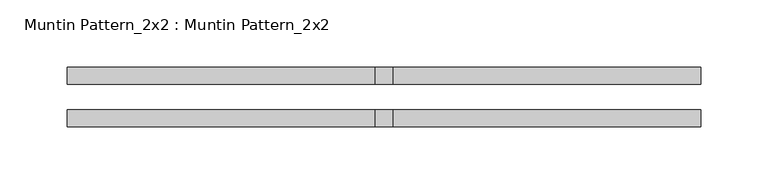
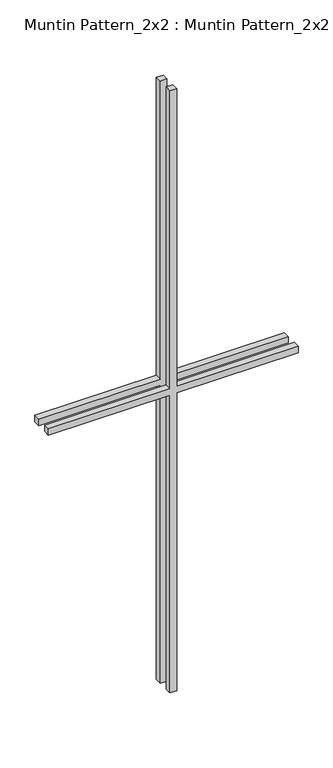
"""IFC4 building model written with IfcOpenShell, lengths in millimetres: proxy geometry, Muntin Pattern_2x2 : Muntin Pattern_2x2."""

from ifc_helpers import new_model, si_unit, frame, origin, place, context, project, spatial, polyline, outline, extrude, source, transform, mapped, element, save


def muntin_pattern_2x2_muntin_pattern_2x2_ba8901dc(model_context):
    return source(origin(), model_context, "Body", "SweptSolid", [
        extrude(outline(polyline([(609.6, -6.35), (609.6, -236.5375), (596.9, -236.5375), (596.9, -6.35), (0.0, -6.35), (0.0, 6.35), (596.9, 6.35), (596.9, 236.5375), (609.6, 236.5375), (609.6, 6.35), (1206.5, 6.35), (1206.5, -6.35), (609.6, -6.35)])), frame((0.0, 9.525, 0.0), z_axis=(0.0, 1.0, 0.0), x_axis=(0.0, 0.0, 1.0)), (0.0, 0.0, 1.0), 12.7),
        extrude(outline(polyline([(609.6, -6.35), (609.6, -236.5375), (596.9, -236.5375), (596.9, -6.35), (0.0, -6.35), (0.0, 6.35), (596.9, 6.35), (596.9, 236.5375), (609.6, 236.5375), (609.6, 6.35), (1206.5, 6.35), (1206.5, -6.35), (609.6, -6.35)])), frame((0.0, -22.225, 0.0), z_axis=(0.0, 1.0, 0.0), x_axis=(0.0, 0.0, 1.0)), (0.0, 0.0, 1.0), 12.7),
    ])


if __name__ == "__main__":
    model = new_model("IFC4")
    model_context = context("Model", 3, world=origin())
    ifc_project = project(units=[si_unit("LENGTHUNIT", "METRE", prefix="MILLI")], contexts=[model_context])
    site = spatial("IfcSite", under=ifc_project)
    building = spatial("IfcBuilding", under=site)
    placement = place(None, origin())
    muntin_pattern_2x2_muntin_pattern_2x2_shape = muntin_pattern_2x2_muntin_pattern_2x2_ba8901dc(model_context)
    element("IfcBuildingElementProxy", 1, Name="Muntin Pattern_2x2 : Muntin Pattern_2x2", ObjectType="Muntin Pattern_2x2 : Muntin Pattern_2x2", at=placement, inside=building, context=model_context, shape_type="MappedRepresentation", body=[
        mapped(muntin_pattern_2x2_muntin_pattern_2x2_shape, transform((0.0, 0.0, 0.0), x_axis=(1.0, 0.0, 0.0), y_axis=(0.0, 1.0, 0.0), z_axis=(0.0, 0.0, 1.0))),
    ])
    save(model, "model.ifc")

# Revit data of these elements
# Type "Muntin Pattern_2x2 : Muntin Pattern_2x2"
#   Width [instance default] = 4' - 0"
#   Thickness = 0' - 0 1/2"
#   Height [instance default] = 4' - 0"
#   Distance = 0' - 0 3/4"
#   Interior Material [instance default] = none
#   Exterior Material [instance default] = none
#   Default Elevation = 0
# Element 1 (IfcBuildingElementProxy, "Muntin Pattern_2x2 : Muntin Pattern_2x2")
#   Width = 1' - 6 5/8"
#   Height = 3' - 11 1/2"
#   Interior Material = Wood - Stained
#   Exterior Material = Clad - White
#   Materials on its faces: "Clad - White", "Wood - Stained"
# Materials
#   "Clad - White": class "Wood", colour RGB 242 242 238, transparency 0, Cost = 0
#   "Wood - Stained": class "Wood", colour RGB 224 178 126, transparency 0, Cost = 0
